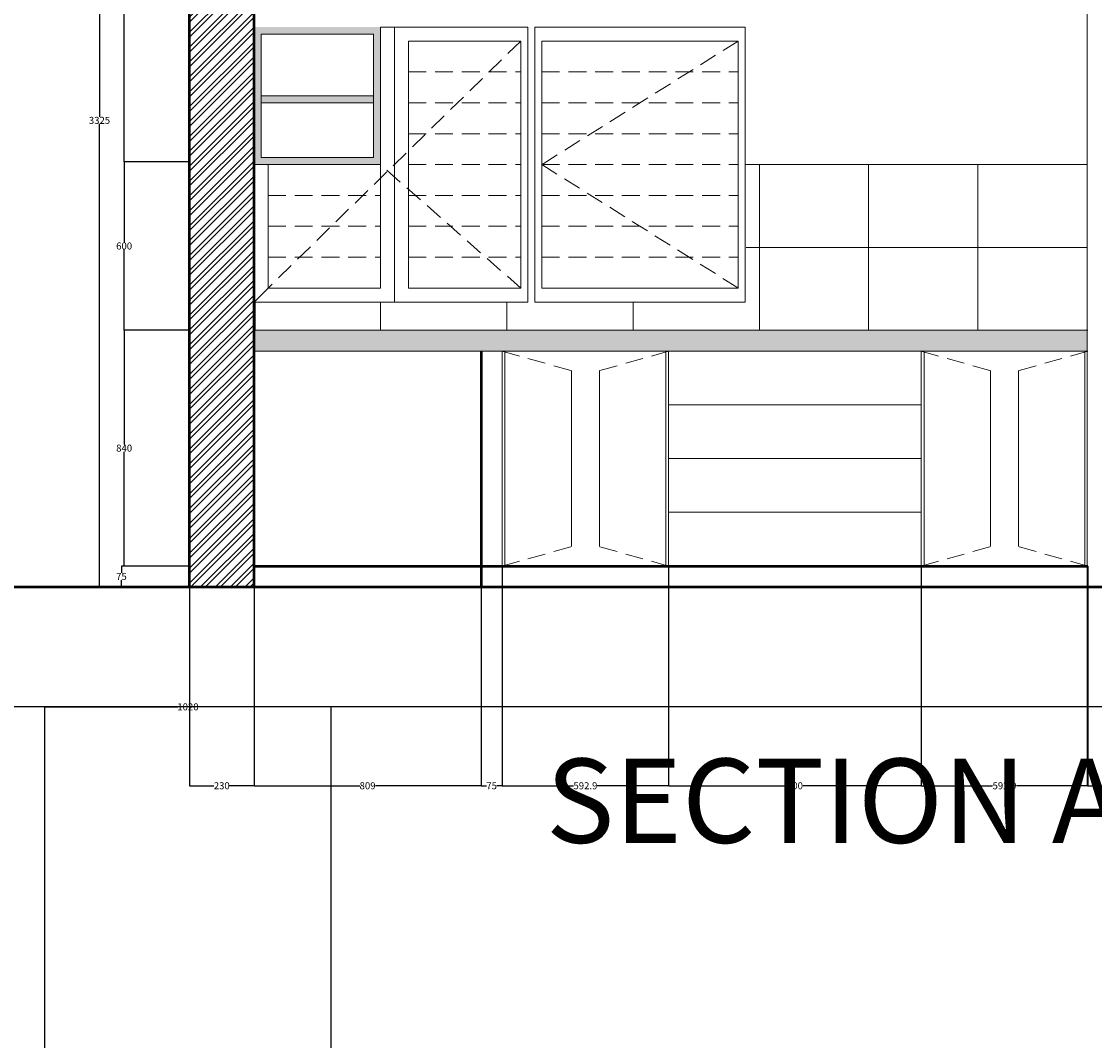
# Model space of a CAD drawing. Units: millimetres. Extents: x 1944 to 29915, y -10550 to 5909.
# Tile 22 of 24: x 19652 to 23475, y -1584 to 2046. Entities that reach past the tile are written whole.
import ezdxf

# ---------------------------------------------------------------- set-up
doc = ezdxf.new("R2010")
doc.units = ezdxf.units.MM
doc.header["$MEASUREMENT"] = 0
doc.linetypes.add('HIDDEN', pattern=[9.525, 6.35, -3.175])
for name, color, linetype, lineweight in [('A-ANNO-DIMS', 2, 'Continuous', 18), ('A-ANNO-TEXT', 7, 'Continuous', 25), ('A-ELEV', 3, 'Continuous', 18), ('A-ELEV-HIDN', 3, 'HIDDEN', 13), ('A-WALL', 7, 'Continuous', 50), ('A-WALL-PATT', 8, 'Continuous', 18)]:
    doc.layers.add(name, color=color, linetype=linetype, lineweight=lineweight)
doc.styles.get("Standard").update_dxf_attribs({"font": 'arial.ttf'})
doc.dimstyles.get("Standard").update_dxf_attribs({"dimtxt": 25, "dimasz": 0.18, "dimexe": 0.18, "dimexo": 0.0625, "dimgap": 0.09, "dimtad": 0, "dimtih": 1, "dimtoh": 1, "dimdec": 0, "dimzin": 0, "dimdsep": 46, "dimtxsty": 'Standard', "dimcen": 0.09, "dimadec": 0, "dimazin": 0, "dimtfac": 1, "dimtdec": 0, "dimtofl": 0, "dimtmove": 0, "dimatfit": 3, "dimfxl": 1, "dimtolj": 1, "dimtzin": 0, "dimarcsym": 0})

# ---------------------------------------------------------------- blocks, each defined once
blk = doc.blocks.new('*D15')
at = {"layer": 'A-ANNO-DIMS', "color": 0, "lineweight": -2, "transparency": 16777216}
for p, q in [((20061.5, 105.8), (20008.5, 105.8)), ((20008.6, 105.7), (20008.6, 81.1)), ((20008.6, 31), (20008.6, 55.5)), ((20061.5, 30.8), (20008.5, 30.8))]:
    blk.add_line(p, q, dxfattribs=at)
at = {"layer": 'A-ANNO-DIMS', "color": 0, "transparency": 16777216}
for points in [[(20008.6, 105.7), (20008.7, 105.7), (20008.6, 105.8)], [(20008.6, 31), (20008.7, 31), (20008.6, 30.8)]]:
    blk.add_solid(points, dxfattribs=at)
at = {"layer": 'Defpoints', "color": 0, "transparency": 16777216}
for p in [(20008.6, 105.8), (20061.5, 105.8), (20061.5, 30.8)]:
    blk.add_point(p, dxfattribs=at)
at = {"layer": 'A-ANNO-DIMS', "color": 0, "transparency": 16777216, "insert": (20008.6, 68.3), "char_height": 25, "attachment_point": 5}
blk.add_mtext('\\A1;75', dxfattribs=at)
blk = doc.blocks.new('*D16')
at = {"layer": 'A-ANNO-DIMS', "color": 0, "lineweight": -2, "transparency": 16777216}
for p, q in [((20250.8, 945.8), (20018.1, 945.8)), ((20018.3, 945.7), (20018.3, 538.7)), ((20018.3, 106), (20018.3, 513)), ((20250.8, 105.8), (20018.1, 105.8))]:
    blk.add_line(p, q, dxfattribs=at)
at = {"layer": 'A-ANNO-DIMS', "color": 0, "transparency": 16777216}
for points in [[(20018.2, 945.7), (20018.3, 945.7), (20018.3, 945.8)], [(20018.2, 106), (20018.3, 106), (20018.3, 105.8)]]:
    blk.add_solid(points, dxfattribs=at)
at = {"layer": 'Defpoints', "color": 0, "transparency": 16777216}
for p in [(20018.3, 945.8), (20250.9, 945.8), (20250.9, 105.8)]:
    blk.add_point(p, dxfattribs=at)
at = {"layer": 'A-ANNO-DIMS', "color": 0, "transparency": 16777216, "insert": (20018.3, 525.8), "char_height": 25, "attachment_point": 5}
blk.add_mtext('\\A1;840', dxfattribs=at)
blk = doc.blocks.new('*D17')
at = {"layer": 'A-ANNO-DIMS', "color": 0, "lineweight": -2, "transparency": 16777216}
for p, q in [((20250.8, 1545.8), (20018.1, 1545.8)), ((20018.2, 1545.7), (20018.2, 1258.7)), ((20018.2, 946), (20018.2, 1233)), ((20250.8, 945.8), (20018.1, 945.8))]:
    blk.add_line(p, q, dxfattribs=at)
at = {"layer": 'A-ANNO-DIMS', "color": 0, "transparency": 16777216}
for points in [[(20018.2, 1545.7), (20018.3, 1545.7), (20018.2, 1545.8)], [(20018.2, 946), (20018.3, 946), (20018.2, 945.8)]]:
    blk.add_solid(points, dxfattribs=at)
at = {"layer": 'Defpoints', "color": 0, "transparency": 16777216}
for p in [(20018.2, 1545.8), (20250.9, 1545.8), (20250.9, 945.8)]:
    blk.add_point(p, dxfattribs=at)
at = {"layer": 'A-ANNO-DIMS', "color": 0, "transparency": 16777216, "insert": (20018.2, 1245.8), "char_height": 25, "attachment_point": 5}
blk.add_mtext('\\A1;600', dxfattribs=at)
blk = doc.blocks.new('*D18')
at = {"layer": 'A-ANNO-DIMS', "color": 0, "lineweight": -2, "transparency": 16777216}
for p, q in [((20250.8, 2905.8), (20018.1, 2905.8)), ((20018.3, 2905.7), (20018.3, 2238.7)), ((20018.3, 1546), (20018.3, 2213)), ((20250.8, 1545.8), (20018.1, 1545.8))]:
    blk.add_line(p, q, dxfattribs=at)
at = {"layer": 'A-ANNO-DIMS', "color": 0, "transparency": 16777216}
for points in [[(20018.2, 2905.7), (20018.3, 2905.7), (20018.3, 2905.8)], [(20018.2, 1546), (20018.3, 1546), (20018.3, 1545.8)]]:
    blk.add_solid(points, dxfattribs=at)
at = {"layer": 'Defpoints', "color": 0, "transparency": 16777216}
for p in [(20018.3, 2905.8), (20250.9, 2905.8), (20250.9, 1545.8)]:
    blk.add_point(p, dxfattribs=at)
at = {"layer": 'A-ANNO-DIMS', "color": 0, "transparency": 16777216, "insert": (20018.3, 2225.8), "char_height": 25, "attachment_point": 5}
blk.add_mtext('\\A1;1360', dxfattribs=at)
blk = doc.blocks.new('*D21')
at = {"layer": 'A-ANNO-DIMS', "color": 0, "lineweight": -2, "transparency": 16777216}
for p, q in [((20124.6, 3355.8), (19930.2, 3355.8)), ((19930.3, 3355.7), (19930.3, 1706.2)), ((19930.3, 31), (19930.3, 1680.5)), ((20061.5, 30.8), (19930.2, 30.8))]:
    blk.add_line(p, q, dxfattribs=at)
at = {"layer": 'A-ANNO-DIMS', "color": 0, "transparency": 16777216}
for points in [[(19930.3, 3355.7), (19930.4, 3355.7), (19930.3, 3355.8)], [(19930.3, 31), (19930.4, 31), (19930.3, 30.8)]]:
    blk.add_solid(points, dxfattribs=at)
at = {"layer": 'Defpoints', "color": 0, "transparency": 16777216}
for p in [(20124.6, 3355.8), (19930.3, 30.8), (20061.5, 30.8)]:
    blk.add_point(p, dxfattribs=at)
at = {"layer": 'A-ANNO-DIMS', "color": 0, "transparency": 16777216, "insert": (19930.3, 1693.3), "char_height": 25, "attachment_point": 5}
blk.add_mtext('\\A1;3325', dxfattribs=at)
blk = doc.blocks.new('*D75')
at = {"layer": 'A-ANNO-DIMS', "color": 0, "lineweight": -2, "transparency": 16777216}
for p, q in [((20250.9, 30.8), (20250.9, -677)), ((20480.9, 30.8), (20480.9, -677)), ((20251, -676.8), (20338, -676.8)), ((20480.7, -676.8), (20393.7, -676.8))]:
    blk.add_line(p, q, dxfattribs=at)
at = {"layer": 'A-ANNO-DIMS', "color": 0, "transparency": 16777216}
for points in [[(20251, -676.8), (20251, -676.9), (20250.9, -676.8)], [(20480.7, -676.8), (20480.7, -676.9), (20480.9, -676.8)]]:
    blk.add_solid(points, dxfattribs=at)
at = {"layer": 'Defpoints', "color": 0, "transparency": 16777216}
for p in [(20250.9, 30.8), (20480.9, 30.8), (20480.9, -676.8)]:
    blk.add_point(p, dxfattribs=at)
at = {"layer": 'A-ANNO-DIMS', "color": 0, "transparency": 16777216, "insert": (20365.9, -676.8), "char_height": 25, "attachment_point": 5}
blk.add_mtext('\\A1;230', dxfattribs=at)
blk = doc.blocks.new('*D76')
at = {"layer": 'A-ANNO-DIMS', "color": 0, "lineweight": -2, "transparency": 16777216}
for p, q in [((20480.9, 105.8), (20480.9, -677)), ((21289.8, 30.8), (21289.8, -677)), ((20481, -676.8), (20857.6, -676.8)), ((21289.6, -676.8), (20913.1, -676.8))]:
    blk.add_line(p, q, dxfattribs=at)
at = {"layer": 'A-ANNO-DIMS', "color": 0, "transparency": 16777216}
for points in [[(20481, -676.8), (20481, -676.9), (20480.9, -676.8)], [(21289.6, -676.8), (21289.6, -676.9), (21289.8, -676.8)]]:
    blk.add_solid(points, dxfattribs=at)
at = {"layer": 'Defpoints', "color": 0, "transparency": 16777216}
for p in [(20480.9, 105.8), (21289.8, 30.8), (21289.8, -676.8)]:
    blk.add_point(p, dxfattribs=at)
at = {"layer": 'A-ANNO-DIMS', "color": 0, "transparency": 16777216, "insert": (20885.3, -676.8), "char_height": 25, "attachment_point": 5}
blk.add_mtext('\\A1;809', dxfattribs=at)
blk = doc.blocks.new('*D77')
at = {"layer": 'A-ANNO-DIMS', "color": 0, "lineweight": -2, "transparency": 16777216}
for p, q in [((21364.8, 105.8), (21364.8, -677)), ((21289.8, 30.8), (21289.8, -677)), ((21290, -676.8), (21309.3, -676.8)), ((21364.6, -676.8), (21345.3, -676.8))]:
    blk.add_line(p, q, dxfattribs=at)
at = {"layer": 'A-ANNO-DIMS', "color": 0, "transparency": 16777216}
for points in [[(21290, -676.8), (21290, -676.9), (21289.8, -676.8)], [(21364.6, -676.8), (21364.6, -676.9), (21364.8, -676.8)]]:
    blk.add_solid(points, dxfattribs=at)
at = {"layer": 'Defpoints', "color": 0, "transparency": 16777216}
for p in [(21364.8, 105.8), (21289.8, 30.8), (21364.8, -676.8)]:
    blk.add_point(p, dxfattribs=at)
at = {"layer": 'A-ANNO-DIMS', "color": 0, "transparency": 16777216, "insert": (21327.3, -676.8), "char_height": 25, "attachment_point": 5}
blk.add_mtext('\\A1;75', dxfattribs=at)
blk = doc.blocks.new('*D78')
at = {"layer": 'A-ANNO-DIMS', "color": 0, "lineweight": -2, "transparency": 16777216}
for p, q in [((21364.8, 105.8), (21364.8, -677)), ((21957.7, 105.8), (21957.7, -677)), ((21365, -676.8), (21619, -676.8)), ((21957.6, -676.8), (21703.6, -676.8))]:
    blk.add_line(p, q, dxfattribs=at)
at = {"layer": 'A-ANNO-DIMS', "color": 0, "transparency": 16777216}
for points in [[(21365, -676.8), (21365, -676.9), (21364.8, -676.8)], [(21957.6, -676.8), (21957.6, -676.9), (21957.7, -676.8)]]:
    blk.add_solid(points, dxfattribs=at)
at = {"layer": 'Defpoints', "color": 0, "transparency": 16777216}
for p in [(21364.8, 105.8), (21957.7, 105.8), (21957.7, -676.8)]:
    blk.add_point(p, dxfattribs=at)
at = {"layer": 'A-ANNO-DIMS', "color": 0, "transparency": 16777216, "insert": (21661.3, -676.8), "char_height": 25, "attachment_point": 5}
blk.add_mtext('\\A1;592.9', dxfattribs=at)
blk = doc.blocks.new('*D79')
at = {"layer": 'A-ANNO-DIMS', "color": 0, "lineweight": -2, "transparency": 16777216}
for p, q in [((21957.7, 105.8), (21957.7, -677)), ((22857.7, 105.8), (22857.7, -677)), ((21957.9, -676.8), (22380.1, -676.8)), ((22857.6, -676.8), (22435.4, -676.8))]:
    blk.add_line(p, q, dxfattribs=at)
at = {"layer": 'A-ANNO-DIMS', "color": 0, "transparency": 16777216}
for points in [[(21957.9, -676.8), (21957.9, -676.9), (21957.7, -676.8)], [(22857.6, -676.8), (22857.6, -676.9), (22857.7, -676.8)]]:
    blk.add_solid(points, dxfattribs=at)
at = {"layer": 'Defpoints', "color": 0, "transparency": 16777216}
for p in [(21957.7, 105.8), (22857.7, 105.8), (22857.7, -676.8)]:
    blk.add_point(p, dxfattribs=at)
at = {"layer": 'A-ANNO-DIMS', "color": 0, "transparency": 16777216, "insert": (22407.7, -676.8), "char_height": 25, "attachment_point": 5}
blk.add_mtext('\\A1;900', dxfattribs=at)
blk = doc.blocks.new('*D80')
at = {"layer": 'A-ANNO-DIMS', "color": 0, "lineweight": -2, "transparency": 16777216}
for p, q in [((22857.7, 105.8), (22857.7, -677)), ((23450.7, 105.8), (23450.7, -677)), ((22857.9, -676.8), (23111.9, -676.8)), ((23450.5, -676.8), (23196.5, -676.8))]:
    blk.add_line(p, q, dxfattribs=at)
at = {"layer": 'A-ANNO-DIMS', "color": 0, "transparency": 16777216}
for points in [[(22857.9, -676.8), (22857.9, -676.9), (22857.7, -676.8)], [(23450.5, -676.8), (23450.5, -676.9), (23450.7, -676.8)]]:
    blk.add_solid(points, dxfattribs=at)
at = {"layer": 'Defpoints', "color": 0, "transparency": 16777216}
for p in [(22857.7, 105.8), (23450.7, 105.8), (23450.7, -676.8)]:
    blk.add_point(p, dxfattribs=at)
at = {"layer": 'A-ANNO-DIMS', "color": 0, "transparency": 16777216, "insert": (23154.2, -676.8), "char_height": 25, "attachment_point": 5}
blk.add_mtext('\\A1;592.9', dxfattribs=at)
blk = doc.blocks.new('*D81')
at = {"layer": 'A-ANNO-DIMS', "color": 0, "lineweight": -2, "transparency": 16777216}
for p, q in [((23449.1, 30.8), (23449.1, -677)), ((24274.1, 30.8), (24274.1, -677)), ((23449.3, -676.8), (23833.8, -676.8)), ((24274, -676.8), (23889.5, -676.8))]:
    blk.add_line(p, q, dxfattribs=at)
at = {"layer": 'A-ANNO-DIMS', "color": 0, "transparency": 16777216}
for points in [[(23449.3, -676.8), (23449.3, -676.9), (23449.1, -676.8)], [(24274, -676.8), (24274, -676.9), (24274.1, -676.8)]]:
    blk.add_solid(points, dxfattribs=at)
at = {"layer": 'Defpoints', "color": 0, "transparency": 16777216}
for p in [(23449.1, 30.8), (24274.1, 30.8), (24274.1, -676.8)]:
    blk.add_point(p, dxfattribs=at)
at = {"layer": 'A-ANNO-DIMS', "color": 0, "transparency": 16777216, "insert": (23861.6, -676.8), "char_height": 25, "attachment_point": 5}
blk.add_mtext('\\A1;825', dxfattribs=at)
blk = doc.blocks.new('*D85')
at = {"layer": 'A-ANNO-DIMS', "color": 0, "lineweight": -2, "transparency": 16777216}
for p, q in [((6418.3, -1730.7), (6418.3, -395.6)), ((6418.5, -395.8), (15860.3, -395.8)), ((25389.1, -395.8), (15947.3, -395.8)), ((25389.3, -1846.5), (25389.3, -395.6))]:
    blk.add_line(p, q, dxfattribs=at)
at = {"layer": 'A-ANNO-DIMS', "color": 0, "transparency": 16777216}
for points in [[(6418.5, -395.7), (6418.5, -395.8), (6418.3, -395.8)], [(25389.1, -395.7), (25389.1, -395.8), (25389.3, -395.8)]]:
    blk.add_solid(points, dxfattribs=at)
at = {"layer": 'Defpoints', "color": 0, "transparency": 16777216}
for p in [(25389.3, -395.8), (6418.3, -1730.8), (25389.3, -1846.5)]:
    blk.add_point(p, dxfattribs=at)
at = {"layer": 'A-ANNO-DIMS', "color": 0, "transparency": 16777216, "insert": (15903.8, -395.8), "char_height": 25, "attachment_point": 5}
blk.add_mtext('\\A1;18971', dxfattribs=at)
blk = doc.blocks.new('*D96')
at = {"layer": 'A-ANNO-DIMS', "color": 0, "lineweight": -2, "transparency": 16777216}
for p, q in [((19735.4, -3070.7), (19735.4, -395.6)), ((19735.6, -395.8), (20209.2, -395.8)), ((20755.3, -395.8), (20281.6, -395.8)), ((20755.4, -3070.7), (20755.4, -395.6))]:
    blk.add_line(p, q, dxfattribs=at)
at = {"layer": 'A-ANNO-DIMS', "color": 0, "transparency": 16777216}
for points in [[(19735.6, -395.7), (19735.6, -395.8), (19735.4, -395.8)], [(20755.3, -395.7), (20755.3, -395.8), (20755.4, -395.8)]]:
    blk.add_solid(points, dxfattribs=at)
at = {"layer": 'Defpoints', "color": 0, "transparency": 16777216}
for p in [(20755.4, -395.8), (19735.4, -3070.8), (20755.4, -3070.8)]:
    blk.add_point(p, dxfattribs=at)
at = {"layer": 'A-ANNO-DIMS', "color": 0, "transparency": 16777216, "insert": (20245.4, -395.8), "char_height": 25, "attachment_point": 5}
blk.add_mtext('\\A1;1020', dxfattribs=at)

msp = doc.modelspace()

# ---------------------------------------------------------------- hatches: boundary and pattern name
at = {"layer": 'A-ELEV'}
h = msp.add_hatch(color=256, dxfattribs=at)
h.dxf.hatch_style = 1
h.paths.add_polyline_path([(20480.858, 2025.837), (20480.858, 1535.837), (20930.858, 1535.837), (20930.858, 1975.837), (20930.858, 2025.837)])
h.paths.add_polyline_path([(20905.858, 2000.837), (20905.858, 1780.837), (20905.858, 1560.837), (20505.858, 1560.837), (20505.858, 1780.837), (20505.858, 2000.837)], flags=16)
h = msp.add_hatch(color=256, dxfattribs=at)
h.dxf.hatch_style = 1
h.paths.add_polyline_path([(20505.858, 1780.837), (20505.858, 1755.837), (20905.858, 1755.837), (20905.858, 1780.837)])
h = msp.add_hatch(color=256, dxfattribs=at)
h.dxf.hatch_style = 1
h.paths.add_polyline_path([(23449.139, 945.837), (20480.858, 945.837), (20480.858, 870.837), (23449.139, 870.837)])
at = {"layer": 'A-WALL-PATT'}
h = msp.add_hatch(dxfattribs=at)
h.set_pattern_fill('ANSI32', color=256, scale=100)
h.paths.add_polyline_path([(20480.858, 2905.837), (20250.858, 2905.837), (20250.858, 30.837), (20480.858, 30.837)])
h = msp.add_hatch(dxfattribs=at)
h.set_pattern_fill('AR-CONC', color=256, scale=100)
h.paths.add_polyline_path([(21289.825, 105.837), (20480.858, 105.837), (20480.858, 30.837), (21289.825, 30.837)])

# ---------------------------------------------------------------- linework, layer by layer
at = {"layer": 'A-ELEV'}
for p, q in [((20505.858, 2000.837), (20905.858, 2000.837)), ((20505.858, 1780.837), (20505.858, 2000.837)), ((20905.858, 2000.837), (20905.858, 1780.837)), ((20930.858, 2025.837), (20930.858, 2025.837)), ((20930.858, 2025.837), (21455.858, 2025.837)), ((20980.858, 1045.837), (20980.858, 2025.837)), ((21455.858, 2025.837), (21455.858, 1045.837)), ((21480.858, 2025.837), (21480.858, 1045.837)), ((21480.858, 2025.837), (21480.858, 1045.837)), ((21480.858, 2025.837), (22230.858, 2025.837)), ((22230.858, 2025.837), (22230.858, 1045.837)), ((22230.858, 2025.837), (22230.858, 1045.837)), ((22205.858, 1975.837), (22205.858, 1095.837)), ((20905.858, 1780.837), (20505.858, 1780.837)), ((20505.858, 1780.837), (20505.858, 1560.837)), ((20905.858, 1780.837), (20905.858, 1560.837)), ((20905.858, 1755.837), (20505.858, 1755.837)), ((20905.858, 1560.837), (20505.858, 1560.837)), ((20530.858, 1535.837), (20930.858, 1535.837)), ((22230.858, 1535.837), (23449.139, 1535.837)), ((22280.858, 945.837), (22280.858, 1535.837)), ((22670.285, 945.837), (22670.285, 1535.837)), ((23059.712, 945.837), (23059.712, 1535.837)), ((23449.139, 945.837), (23449.139, 1535.837)), ((22234.186, 1240.837), (23449.139, 1240.837)), ((20530.858, 1095.837), (20480.858, 1045.837)), ((20480.858, 1045.837), (21455.858, 1045.837)), ((20930.858, 1045.837), (20930.858, 945.837)), ((20930.858, 1045.837), (20930.858, 945.837)), ((21380.858, 1045.837), (21380.858, 945.837)), ((21380.858, 1045.837), (21380.858, 945.837)), ((21480.858, 1045.837), (22230.858, 1045.837)), ((21830.858, 1045.837), (21830.858, 945.837)), ((21830.858, 1045.837), (21830.858, 945.837)), ((20480.858, 945.837), (23450.661, 945.837)), ((20480.858, 870.837), (23450.661, 870.837)), ((21364.825, 870.837), (21364.825, 105.837)), ((21374.825, 870.837), (21374.825, 105.837)), ((21947.743, 870.837), (21947.743, 105.837)), ((21957.743, 870.837), (22857.743, 870.837)), ((22857.743, 870.837), (22857.743, 105.837)), ((22867.743, 870.837), (22867.743, 105.837)), ((23440.661, 870.837), (23440.661, 105.837)), ((21611.284, 801.845), (21611.284, 174.829)), ((21711.284, 801.845), (21711.284, 174.829)), ((23104.202, 801.845), (23104.202, 174.829)), ((23204.202, 801.845), (23204.202, 174.829)), ((21957.743, 679.587), (22857.743, 679.587)), ((21957.743, 488.337), (22857.743, 488.337)), ((21957.743, 297.087), (22857.743, 297.087)), ((21957.743, 105.837), (22857.743, 105.837))]:
    msp.add_line(p, q, dxfattribs=at)
for points in [[(23449.139, 30.837), (23449.139, 2905.837), (24249.139, 2905.837)], [(20930.858, 2025.837), (20930.858, 1975.837)], [(20930.858, 1975.837), (20930.858, 1095.837), (20530.858, 1095.837), (20530.858, 1535.837)], [(20930.858, 1535.837), (20480.858, 1535.837)]]:
    msp.add_lwpolyline(points, dxfattribs=at)
for points in [[(21030.858, 1975.837), (21430.858, 1975.837), (21430.858, 1095.837), (21030.858, 1095.837)], [(21505.858, 1975.837), (22205.858, 1975.837), (22205.858, 1095.837), (21505.858, 1095.837)], [(21364.825, 870.837), (21957.743, 870.837), (21957.743, 105.837), (21364.825, 105.837)]]:
    msp.add_lwpolyline(points, close=True, dxfattribs=at)
at = {"layer": 'A-ELEV-HIDN', "ltscale": 10}
for p, q in [((21430.858, 1975.837), (20530.858, 1095.837)), ((22205.858, 1975.837), (21505.858, 1535.837)), ((21030.858, 1865.837), (21430.858, 1865.837)), ((21505.858, 1865.837), (22205.858, 1865.837)), ((21030.858, 1755.837), (21430.858, 1755.837)), ((21505.858, 1755.837), (22205.858, 1755.837)), ((21030.858, 1645.837), (21430.858, 1645.837)), ((21505.858, 1645.837), (22205.858, 1645.837)), ((21430.858, 1095.837), (20930.858, 1535.837)), ((21030.858, 1535.837), (21430.858, 1535.837)), ((21505.858, 1535.837), (22205.858, 1535.837)), ((21505.858, 1535.837), (22205.858, 1095.837)), ((20530.858, 1425.837), (20930.858, 1425.837)), ((21030.858, 1425.837), (21430.858, 1425.837)), ((21505.858, 1425.837), (22205.858, 1425.837)), ((20530.858, 1315.837), (20930.858, 1315.837)), ((21030.858, 1315.837), (21430.858, 1315.837)), ((21505.858, 1315.837), (22205.858, 1315.837)), ((20530.858, 1205.837), (20930.858, 1205.837)), ((21030.858, 1205.837), (21430.858, 1205.837)), ((21505.858, 1205.837), (22205.858, 1205.837)), ((21364.825, 870.837), (21611.284, 801.845)), ((21957.743, 870.837), (21711.284, 801.845)), ((22857.743, 870.837), (23104.202, 801.845)), ((23450.661, 870.837), (23204.202, 801.845)), ((21364.825, 105.837), (21611.284, 174.829)), ((21957.743, 105.837), (21711.284, 174.829)), ((22857.743, 105.837), (23104.202, 174.829)), ((23450.661, 105.837), (23204.202, 174.829))]:
    msp.add_line(p, q, dxfattribs=at)
at = {"layer": 'A-WALL'}
for p, q in [((20250.858, 30.837), (20250.858, 3230.837)), ((20480.858, 30.837), (20480.858, 3230.837)), ((20480.858, 1045.837), (20480.858, 945.837)), ((21289.825, 870.837), (21289.825, 30.837)), ((20480.858, 105.837), (23450.661, 105.837)), ((24504.139, 30.837), (12776.548, 30.837))]:
    msp.add_line(p, q, dxfattribs=at)

# ---------------------------------------------------------------- texts
at = {"layer": 'A-ANNO-TEXT'}
msp.add_text("SECTION AT 'B'", height=300, dxfattribs=at).set_placement((21520.494, -880.236))

# ---------------------------------------------------------------- dimensions: what is measured, and where the dimension line sits
at = {"layer": 'A-ANNO-DIMS'}
for base, p1, p2, picture, middle in [((19930.341, 30.837), (20124.649, 3355.837), (20061.543, 30.837), '*D21', (19930.341, 1693.337)), ((20018.27, 2905.837), (20250.858, 1545.837), (20250.858, 2905.837), '*D18', (20018.27, 2225.837)), ((20018.24, 1545.837), (20250.858, 945.837), (20250.858, 1545.837), '*D17', (20018.24, 1245.837)), ((20018.27, 945.837), (20250.858, 105.837), (20250.858, 945.837), '*D16', (20018.27, 525.837)), ((20008.642, 105.837), (20061.543, 30.837), (20061.543, 105.837), '*D15', (20008.642, 68.337))]:
    dim = msp.add_linear_dim(base=base, p1=p1, p2=p2, angle=90, dimstyle='Standard', override={"dimclrd": 0, "dimclre": 0, "dimclrt": 0}, dxfattribs=at)
    dim.commit()
    dim.dimension.update_dxf_attribs({"geometry": picture, "text_midpoint": middle})
for base, p1, p2, override, picture, middle in [((21289.825, -676.843), (20480.858, 105.837), (21289.825, 30.837), {"dimdec": 0, "dimlfac": 1, "dimrnd": 0, "dimzin": 0, "dimdsep": 46, "dimlunit": 2}, '*D76', (20885.341, -676.843)), ((21364.825, -676.843), (21289.825, 30.837), (21364.825, 105.837), {"dimdec": 0, "dimlfac": 1, "dimrnd": 0, "dimzin": 0, "dimdsep": 46, "dimlunit": 2}, '*D77', (21327.325, -676.843)), ((21957.743, -676.843), (21364.825, 105.837), (21957.743, 105.837), {"dimdec": 1, "dimlfac": 1, "dimrnd": 0, "dimzin": 0, "dimdsep": 46, "dimlunit": 2}, '*D78', (21661.284, -676.843)), ((22857.743, -676.843), (21957.743, 105.837), (22857.743, 105.837), {"dimdec": 0, "dimlfac": 1, "dimrnd": 0, "dimzin": 0, "dimdsep": 46, "dimlunit": 2}, '*D79', (22407.743, -676.843)), ((23450.661, -676.843), (22857.743, 105.837), (23450.661, 105.837), {"dimdec": 1, "dimlfac": 1, "dimrnd": 0, "dimzin": 0, "dimdsep": 46, "dimlunit": 2}, '*D80', (23154.202, -676.843)), ((20480.858, -676.843), (20250.858, 30.837), (20480.858, 30.837), {"dimdec": 0, "dimlfac": 1, "dimrnd": 0, "dimzin": 0, "dimdsep": 46, "dimlunit": 2}, '*D75', (20365.858, -676.843)), ((24274.139, -676.843), (23449.139, 30.837), (24274.139, 30.837), {"dimdec": 0, "dimlfac": 1, "dimrnd": 0, "dimzin": 0, "dimdsep": 46, "dimlunit": 2}, '*D81', (23861.639, -676.843)), ((25389.297, -395.752), (6418.315, -1730.752), (25389.297, -1846.542), {"dimdec": 0, "dimlfac": 1, "dimrnd": 0, "dimzin": 0, "dimdsep": 46, "dimlunit": 2}, '*D85', (15903.806, -395.752)), ((20755.45, -395.752), (19735.45, -3070.752), (20755.45, -3070.752), {"dimdec": 0, "dimlfac": 1, "dimrnd": 0, "dimzin": 0, "dimdsep": 46, "dimlunit": 2}, '*D96', (20245.45, -395.752))]:
    dim = msp.add_linear_dim(base=base, p1=p1, p2=p2, dimstyle='Standard', override=override, dxfattribs=at)
    dim.commit()
    dim.dimension.update_dxf_attribs({"geometry": picture, "text_midpoint": middle})

doc.saveas('drawing.dxf')
